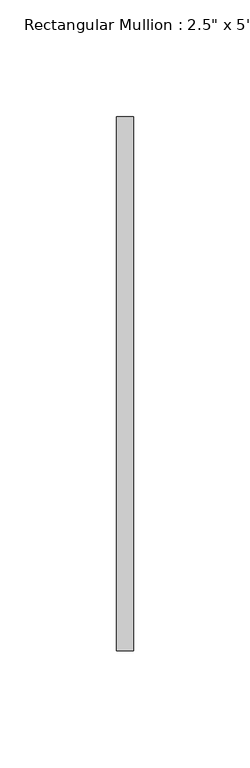
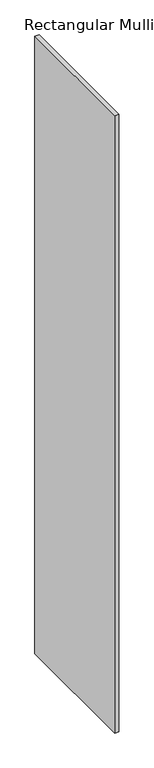
"""IFC4 building model written with IfcOpenShell, lengths in millimetres: member geometry."""

from ifc_helpers import new_model, si_unit, frame, origin, place, context, project, spatial, polyline, outline, extrude, source, transform, mapped, element, save


def member_06a73730(model_context):
    return source(origin(), model_context, "Body", "SweptSolid", [
        extrude(outline(polyline([(3.6195, 114.3), (3.6195, -114.3), (-3.6195, -114.3), (-3.6195, 114.3), (3.6195, 114.3)])), frame((0.0, 0.0, -1081.3415), z_axis=(0.0, 0.0, 1.0), x_axis=(1.0, 0.0, 0.0)), (0.0, 0.0, 1.0), 1081.3415),
    ])


if __name__ == "__main__":
    model = new_model("IFC4")
    model_context = context("Model", 3, world=origin())
    ifc_project = project(units=[si_unit("LENGTHUNIT", "METRE", prefix="MILLI")], contexts=[model_context])
    site = spatial("IfcSite", under=ifc_project)
    building = spatial("IfcBuilding", under=site)
    placement = place(None, origin())
    member_shape = member_06a73730(model_context)
    element("IfcMember", 1, ObjectType="Rectangular Mullion : 2.5\" x 5\" rectangular", at=placement, inside=building, context=model_context, shape_type="MappedRepresentation", body=[
        mapped(member_shape, transform((0.0, 0.0, 0.0), x_axis=(1.0, 0.0, 0.0), y_axis=(0.0, 1.0, 0.0), z_axis=(0.0, 0.0, 1.0))),
    ])
    save(model, "model.ifc")

# Revit data of these elements
# Type "Rectangular Mullion : 2.5\" x 5\" rectangular"
#   built-in parameter 1007304 = 0.75 (stored number, unit not read)
#   built-in parameter 1007301 = 0.011875 (stored number, unit not read)
#   built-in parameter 1007300 = 0.011875 (stored number, unit not read)
# Element 1 (IfcMember, "Rectangular Mullion : 2.5\" x 5\" rectangular")
#   Materials on its faces: "WINDOW GLASS MATERIAL"
# Materials
#   "WINDOW GLASS MATERIAL": class "Generic", colour RGB 120 120 120, transparency 0, Cost = 0
